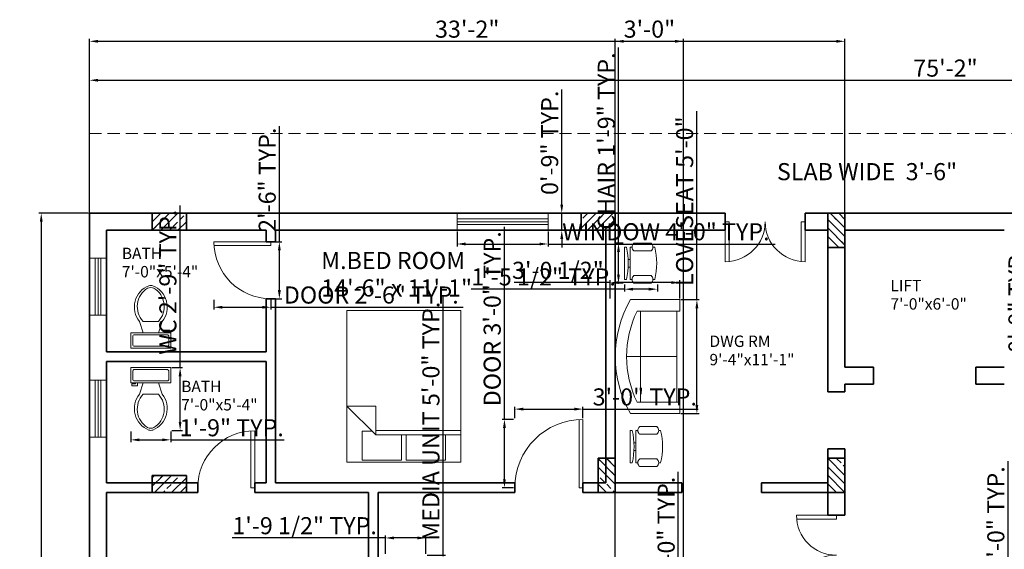
# Model space of a CAD drawing. Units: inches. Extents: x 2081 to 4786, y 1256 to 3802.
# Tile 5 of 7: x 2166 to 2685, y 1804 to 2083. Entities that reach past the tile are written whole.
import ezdxf

# ---------------------------------------------------------------- set-up
doc = ezdxf.new("R2010")
doc.units = ezdxf.units.IN
doc.linetypes.add('HIDDEN', pattern=[9.525, 6.35, -3.175])
for name, color, linetype, lineweight in [('A-ANNO-DIMS', 18, 'Continuous', 18), ('A-ANNO-TEXT', 18, 'Continuous', 18), ('A-AREA-IDEN', 18, 'Continuous', 18), ('A-COLS', 1, 'Continuous', 35), ('A-COLS-PATT', 1, 'Continuous', 13), ('A-DOOR', 5, 'Continuous', 18), ('A-FLOR-FIXT', 18, 'Continuous', 18), ('A-FLOR-OVHD', 18, 'HIDDEN', 18), ('A-FURN', 5, 'Continuous', 18), ('A-GLAZ', 11, 'Continuous', 18), ('A-WALL', 7, 'Continuous', 35)]:
    doc.layers.add(name, color=color, linetype=linetype, lineweight=lineweight)
doc.styles.get("Standard").update_dxf_attribs({"font": 'arial.ttf'})
doc.dimstyles.new('ISO-25', dxfattribs={"dimtxt": 9, "dimasz": 4.5, "dimexe": 1.25, "dimexo": 0.625, "dimtad": 1, "dimdec": 0, "dimlunit": 3, "dimtxsty": 'Standard', "dimcen": 2.5, "dimadec": 0, "dimazin": 0, "dimtfac": 1, "dimtdec": 0, "dimtmove": 0, "dimatfit": 3, "dimfxl": 1, "dimarcsym": 0})
pattern_1 = [(45, (-712.752, 64.734), (-13.47038, 13.47038), []), (45, (-708.262, 64.734), (-13.47038, 13.47038), []), (45, (-703.772, 64.734), (-13.47038, 13.47038), []), (45, (-699.281, 64.734), (-13.47038, 13.47038), [])]
pattern_2 = [(135, (1916.44, -3174.735), (-13.47038, -13.47038), []), (135, (1916.44, -3170.245), (-13.47038, -13.47038), []), (135, (1916.44, -3165.755), (-13.47038, -13.47038), []), (135, (1916.44, -3161.265), (-13.47038, -13.47038), [])]

# ---------------------------------------------------------------- blocks, each defined once
blk = doc.blocks.new('Sofa - Roundback Loveseat 5 ft.')
for p, q in [((0, -32.44198), (0, -5.99998)), ((-24, -33.99998), (-24, -11.46958)), ((-23.9998, -13.38178), (23.99986, -13.38178)), ((24.00004, -33.99998), (24.00004, -11.46958)), ((-24, -32.44198), (24.00004, -32.44198))]:
    blk.add_line(p, q)
for points in [[(-24, -33.99998), (-30, -33.99998), (-30, -7.99998)], [(30.00004, -7.99998), (30.00004, -33.99998), (24.00004, -33.99998)]]:
    blk.add_lwpolyline(points)
for centre, radius, start, end in [((0, -60.24998), 60.24998, 60.13715, 119.8628), ((0, -61.38438), 55.38444, 64.32083, 115.6792)]:
    blk.add_arc(centre, radius, start, end)
blk = doc.blocks.new('Bed - Queen')
for p, q in [((0, -80.00003), (0, 0)), ((0, 0), (59.99999, 0)), ((59.99999, 0), (59.99999, -80.00003)), ((7.99999, -1.2), (28.79998, -1.2)), ((7.99999, -14.4), (7.99999, -1.2)), ((28.79998, -1.2), (28.79998, -14.4)), ((31.19999, -1.2), (51.99999, -1.2)), ((31.19999, -14.4), (31.19999, -1.2)), ((51.99999, -1.2), (51.99999, -16.4)), ((0, -14.4), (44.8, -14.4)), ((59.99999, -29.6), (44.8, -14.4)), ((44.8, -14.4), (44.8, -29.6)), ((44.8, -16.8), (0, -16.8)), ((51.99999, -16.4), (46.79936, -16.4)), ((44.8, -29.6), (59.99999, -29.6)), ((59.99999, -80.00003), (0, -80.00003))]:
    blk.add_line(p, q)
blk = doc.blocks.new('Chair - Desk')
for p, q in [((-8.5, 0), (-8.5, -1)), ((-8.5, 0), (8.5, 0)), ((8.5, 0), (8.5, -1)), ((-10.5, -5), (-10.5, -14)), ((-8.5, -3), (-8.5, -4)), ((-8.5, -3), (8.5, -3)), ((-6.5, -14), (-6.5, -5)), ((-2, -3), (-2, -1.9355)), ((2, -1.9576), (2, -3)), ((6.5, -5), (6.5, -14)), ((8.5, -3), (8.5, -4)), ((10.5, -14), (10.5, -5)), ((-8.5, -15), (-8.5, -16)), ((8.5, -15), (8.5, -16))]:
    blk.add_line(p, q)
for centre, radius, start, end in [((-8.5, -6.5), 2.5, 36.8699, 143.1301), ((0, 34.625), 36.625, 256.5803, 283.4197), ((8.5, -6.5), 2.5, 36.8699, 143.1301), ((-8.5, -12.5), 2.5, 216.8699, 323.1301), ((8.5, -12.5), 2.5, 216.8699, 323.1301), ((0, 19.625), 36.625, 256.5803, 283.4197)]:
    blk.add_arc(centre, radius, start, end)
blk = doc.blocks.new('Toilet - top')
for p, q in [((9.5, -6), (9.5, -2)), ((-10, -8.5), (-8, -8.5)), ((-10, -9.5), (-10, -8.5)), ((-7, -9.5), (-10, -9.5)), ((-8, -8.5), (-8, -8)), ((-7, -8), (-7, -9.5)), ((-4, -8), (-6, -14)), ((4, -8), (6, -14)), ((4, -14), (-4, -14))]:
    blk.add_line(p, q)
blk.add_lwpolyline([(10.5, -8), (10.5, 0), (-10.5, 0), (-10.5, -8)], close=True)
for points in [[(-9.5, -2), (-9.5, -6)], [(8.5, -1), (-8.5, -1)], [(-8.5, -7), (8.5, -7)]]:
    blk.add_lwpolyline(points)
for centre, radius, start, end in [((-8.62, -1.88), 0.884, 81.8699, 188.1301), ((8.62, -1.88), 0.884, 351.8699, 98.1301), ((-8.62, -6.12), 0.884, 171.8699, 278.1301), ((8.62, -6.12), 0.884, 261.8699, 8.1301), ((3.52, -21.58), 12.17, 141.4691, 247.9714), ((4.2, -21.82), 11.33, 136.3677, 238.9468), ((-3.52, -21.58), 12.17, 292.0284, 38.5307), ((-4.2, -21.82), 11.33, 301.053, 43.6321), ((0, -27.88), 4, 245.7318, 294.2682), ((0, -29), 4, 254.8605, 285.1395)]:
    blk.add_arc(centre, radius, start, end)
blk = doc.blocks.new('*D23')
at = {"layer": 'A-ANNO-DIMS', "color": 0, "lineweight": -2, "transparency": 16777216}
for p, q in [((2202.98, 2023.8), (2202.98, 2052.41)), ((2207.48, 2051.16), (3100.48, 2051.16)), ((3104.98, 2023.8), (3104.98, 2052.41))]:
    blk.add_line(p, q, dxfattribs=at)
at = {"layer": 'A-ANNO-DIMS', "color": 0, "transparency": 16777216}
for points in [[(2207.48, 2051.91), (2207.48, 2050.41), (2202.98, 2051.16)], [(3100.48, 2051.91), (3100.48, 2050.41), (3104.98, 2051.16)]]:
    blk.add_solid(points, dxfattribs=at)
at = {"layer": 'Defpoints', "color": 0, "transparency": 16777216}
for p in [(3104.98, 2051.16), (2202.98, 2023.17), (3104.98, 2023.17)]:
    blk.add_point(p, dxfattribs=at)
at = {"layer": 'A-ANNO-DIMS', "color": 0, "transparency": 16777216, "insert": (2653.98, 2056.38), "char_height": 9, "attachment_point": 5}
blk.add_mtext('75\'-2"', dxfattribs=at)
blk = doc.blocks.new('*D25')
at = {"layer": 'A-ANNO-DIMS', "color": 0, "lineweight": -2, "transparency": 16777216}
for p, q in [((2202.36, 1981.17), (2176.26, 1981.17)), ((2177.51, 1976.67), (2177.51, 1437.67)), ((2202.36, 1433.17), (2176.26, 1433.17))]:
    blk.add_line(p, q, dxfattribs=at)
at = {"layer": 'A-ANNO-DIMS', "color": 0, "transparency": 16777216}
for points in [[(2176.76, 1976.67), (2178.26, 1976.67), (2177.51, 1981.17)], [(2176.76, 1437.67), (2178.26, 1437.67), (2177.51, 1433.17)]]:
    blk.add_solid(points, dxfattribs=at)
at = {"layer": 'Defpoints', "color": 0, "transparency": 16777216}
for p in [(2202.98, 1981.17), (2177.51, 1433.17), (2202.98, 1433.17)]:
    blk.add_point(p, dxfattribs=at)
at = {"layer": 'A-ANNO-DIMS', "color": 0, "transparency": 16777216, "insert": (2172.29, 1707.17), "char_height": 9, "attachment_point": 5, "rotation": 90}
blk.add_mtext('45\'-8"', dxfattribs=at)
blk = doc.blocks.new('DOOR-PAIR-42IN')
for p, q in [((0, 42), (21, 42)), ((21, 42), (21, 40)), ((0, 40), (21, 40)), ((0, 2), (21, 2)), ((21, 0), (21, 2)), ((0, 0), (21, 0))]:
    blk.add_line(p, q)
for centre, start, end in [((21, 42), 180, 270), ((21, 0), 90, 180)]:
    blk.add_arc(centre, 21, start, end)
blk = doc.blocks.new('DOOR-SINGLE-36IN')
for p, q in [((34, 36), (34, 0)), ((36, 36), (36, 0)), ((36, 0), (34, 0))]:
    blk.add_line(p, q)
blk.add_arc((36, 0), 36, 90, 180)
blk = doc.blocks.new('DOOR-SINGLE-30IN')
for p, q in [((0, 30), (30, 30)), ((0, 28), (30, 28)), ((30, 30), (30, 28))]:
    blk.add_line(p, q)
blk.add_arc((30, 30), 30, 180, 270)
blk = doc.blocks.new('WINDOW-48IN')
for p, q in [((0, 0), (0, 9)), ((0, 9), (4, 9)), ((48, 6), (0, 6)), ((4, 9), (48, 9)), ((48, 0), (48, 9)), ((48, 4.5), (0, 4.5)), ((48, 3), (0, 3)), ((48, 0), (0, 0))]:
    blk.add_line(p, q)
blk = doc.blocks.new('WINDOW-30IN')
for p, q in [((0, 0), (0, 30)), ((0, 30), (9, 30)), ((3, 0), (3, 30)), ((4.5, 0), (4.5, 30)), ((6, 0), (6, 30)), ((9, 30), (9, 0)), ((9, 0), (0, 0))]:
    blk.add_line(p, q)
blk = doc.blocks.new('COLUMN-9X18IN')
h = blk.add_hatch()
h.set_pattern_fill('ANSI34', color=256, angle=90)
h.set_pattern_definition(pattern_2)
h.paths.add_polyline_path([(9, 18), (0, 18), (0, 0), (9, 0)])
h = blk.add_hatch()
h.set_pattern_fill('ANSI34', color=256, angle=90)
h.set_pattern_definition(pattern_2)
h.paths.add_polyline_path([(9, 18), (0, 18), (0, 0), (9, 0)])
h = blk.add_hatch()
h.set_pattern_fill('ANSI34', color=256, angle=90)
h.set_pattern_definition(pattern_2)
h.paths.add_polyline_path([(9, 18), (0, 18), (0, 0), (9, 0)])
h = blk.add_hatch()
h.set_pattern_fill('ANSI33', color=256, angle=90)
h.set_pattern_definition([(135, (1916.44, -3174.7355), (-4.490128, -4.490128), []), (135, (1916.44, -3170.2454), (-4.490128, -4.490128), [3.175, -1.5875])])
h.paths.add_polyline_path([(0, 0), (9, 0), (9, 18), (0, 18)])
for p, q in [((0, 0), (0, 18)), ((0, 18), (9, 18)), ((9, 18), (9, 0)), ((9, 0), (0, 0))]:
    blk.add_line(p, q)
blk = doc.blocks.new('*D35')
at = {"layer": 'A-ANNO-DIMS', "color": 0, "lineweight": -2, "transparency": 16777216}
for p, q in [((2396.59, 1971.55), (2396.59, 1963.72)), ((2444.59, 1971.55), (2444.59, 1963.72)), ((2401.09, 1964.97), (2440.09, 1964.97)), ((2444.59, 1964.97), (2564.22, 1964.97))]:
    blk.add_line(p, q, dxfattribs=at)
at = {"layer": 'A-ANNO-DIMS', "color": 0, "transparency": 16777216}
for points in [[(2401.09, 1965.72), (2401.09, 1964.22), (2396.59, 1964.97)], [(2440.09, 1965.72), (2440.09, 1964.22), (2444.59, 1964.97)]]:
    blk.add_solid(points, dxfattribs=at)
at = {"layer": 'Defpoints', "color": 0, "transparency": 16777216}
for p in [(2396.59, 1972.17), (2444.59, 1972.17), (2444.59, 1964.97)]:
    blk.add_point(p, dxfattribs=at)
at = {"layer": 'A-ANNO-DIMS', "color": 0, "transparency": 16777216, "insert": (2506.66, 1970.25), "char_height": 9, "attachment_point": 5}
blk.add_mtext('WINDOW 4\'-0" TYP.', dxfattribs=at)
blk = doc.blocks.new('*D36')
at = {"layer": 'A-ANNO-DIMS', "color": 0, "lineweight": -2, "transparency": 16777216}
for p, q in [((2451.79, 1985.67), (2451.79, 2046.28)), ((2445.21, 1981.17), (2453.04, 1981.17)), ((2451.79, 1972.17), (2451.79, 1981.17)), ((2445.21, 1972.17), (2453.04, 1972.17)), ((2451.79, 1967.67), (2451.79, 1963.17))]:
    blk.add_line(p, q, dxfattribs=at)
at = {"layer": 'A-ANNO-DIMS', "color": 0, "transparency": 16777216}
for points in [[(2451.04, 1985.67), (2452.54, 1985.67), (2451.79, 1981.17)], [(2451.04, 1967.67), (2452.54, 1967.67), (2451.79, 1972.17)]]:
    blk.add_solid(points, dxfattribs=at)
at = {"layer": 'Defpoints', "color": 0, "transparency": 16777216}
for p in [(2444.59, 1981.17), (2451.79, 1981.17), (2444.59, 1972.17)]:
    blk.add_point(p, dxfattribs=at)
at = {"layer": 'A-ANNO-DIMS', "color": 0, "transparency": 16777216, "insert": (2446.57, 2018.23), "char_height": 9, "attachment_point": 5, "rotation": 90}
blk.add_mtext('0\'-9" TYP.', dxfattribs=at)
blk = doc.blocks.new('*D39')
at = {"layer": 'A-ANNO-DIMS', "color": 0, "lineweight": -2, "transparency": 16777216}
for p, q in [((2421.58, 1872.67), (2421.58, 1974.05)), ((2426.36, 1872.67), (2420.33, 1872.67)), ((2421.58, 1841.17), (2421.58, 1868.17)), ((2426.36, 1836.67), (2420.33, 1836.67))]:
    blk.add_line(p, q, dxfattribs=at)
at = {"layer": 'A-ANNO-DIMS', "color": 0, "transparency": 16777216}
for points in [[(2420.83, 1868.17), (2422.33, 1868.17), (2421.58, 1872.67)], [(2420.83, 1841.17), (2422.33, 1841.17), (2421.58, 1836.67)]]:
    blk.add_solid(points, dxfattribs=at)
at = {"layer": 'Defpoints', "color": 0, "transparency": 16777216}
for p in [(2421.58, 1872.67), (2426.98, 1872.67), (2426.98, 1836.67)]:
    blk.add_point(p, dxfattribs=at)
at = {"layer": 'A-ANNO-DIMS', "color": 0, "transparency": 16777216, "insert": (2416.3, 1925.61), "char_height": 9, "attachment_point": 5, "rotation": 90}
blk.add_mtext('DOOR 3\'-0" TYP.', dxfattribs=at)
blk = doc.blocks.new('*D40')
at = {"layer": 'A-ANNO-DIMS', "color": 0, "lineweight": -2, "transparency": 16777216}
for p, q in [((2426.98, 1873.3), (2426.98, 1879.32)), ((2462.98, 1873.3), (2462.98, 1879.32)), ((2431.48, 1878.07), (2458.48, 1878.07)), ((2462.98, 1878.07), (2523.59, 1878.07))]:
    blk.add_line(p, q, dxfattribs=at)
at = {"layer": 'A-ANNO-DIMS', "color": 0, "transparency": 16777216}
for points in [[(2431.48, 1878.82), (2431.48, 1877.32), (2426.98, 1878.07)], [(2458.48, 1878.82), (2458.48, 1877.32), (2462.98, 1878.07)]]:
    blk.add_solid(points, dxfattribs=at)
at = {"layer": 'Defpoints', "color": 0, "transparency": 16777216}
for p in [(2462.98, 1878.07), (2426.98, 1872.67), (2462.98, 1872.67)]:
    blk.add_point(p, dxfattribs=at)
at = {"layer": 'A-ANNO-DIMS', "color": 0, "transparency": 16777216, "insert": (2495.54, 1883.3), "char_height": 9, "attachment_point": 5}
blk.add_mtext('3\'-0" TYP.', dxfattribs=at)
blk = doc.blocks.new('*D41')
at = {"layer": 'A-ANNO-DIMS', "color": 0, "lineweight": -2, "transparency": 16777216}
for p, q in [((2250.68, 1899.88), (2250.68, 1985.3)), ((2246.35, 1899.88), (2251.93, 1899.88)), ((2250.68, 1871.33), (2250.68, 1895.38)), ((2246.35, 1866.83), (2251.93, 1866.83))]:
    blk.add_line(p, q, dxfattribs=at)
at = {"layer": 'A-ANNO-DIMS', "color": 0, "transparency": 16777216}
for points in [[(2249.93, 1895.38), (2251.43, 1895.38), (2250.68, 1899.88)], [(2249.93, 1871.33), (2251.43, 1871.33), (2250.68, 1866.83)]]:
    blk.add_solid(points, dxfattribs=at)
at = {"layer": 'Defpoints', "color": 0, "transparency": 16777216}
for p in [(2245.73, 1899.88), (2250.68, 1899.88), (2245.73, 1866.83)]:
    blk.add_point(p, dxfattribs=at)
at = {"layer": 'A-ANNO-DIMS', "color": 0, "transparency": 16777216, "insert": (2245.4, 1944.84), "char_height": 9, "attachment_point": 5, "rotation": 90}
blk.add_mtext('WC 2\'-9" TYP.', dxfattribs=at)
blk = doc.blocks.new('*D42')
at = {"layer": 'A-ANNO-DIMS', "color": 0, "lineweight": -2, "transparency": 16777216}
for p, q in [((2224.73, 1866.21), (2224.73, 1860.63)), ((2245.73, 1866.21), (2245.73, 1860.63)), ((2229.23, 1861.88), (2241.23, 1861.88)), ((2245.73, 1861.88), (2305.49, 1861.88))]:
    blk.add_line(p, q, dxfattribs=at)
at = {"layer": 'A-ANNO-DIMS', "color": 0, "transparency": 16777216}
for points in [[(2229.23, 1862.63), (2229.23, 1861.13), (2224.73, 1861.88)], [(2241.23, 1862.63), (2241.23, 1861.13), (2245.73, 1861.88)]]:
    blk.add_solid(points, dxfattribs=at)
at = {"layer": 'Defpoints', "color": 0, "transparency": 16777216}
for p in [(2224.73, 1866.83), (2245.73, 1866.83), (2245.73, 1861.88)]:
    blk.add_point(p, dxfattribs=at)
at = {"layer": 'A-ANNO-DIMS', "color": 0, "transparency": 16777216, "insert": (2277.86, 1867.1), "char_height": 9, "attachment_point": 5}
blk.add_mtext('1\'-9" TYP.', dxfattribs=at)
blk = doc.blocks.new('*D45')
at = {"layer": 'A-ANNO-DIMS', "color": 0, "lineweight": -2, "transparency": 16777216}
for p, q in [((2268.48, 1935.55), (2268.48, 1930.42)), ((2298.48, 1935.55), (2298.48, 1930.42)), ((2272.98, 1931.67), (2293.98, 1931.67)), ((2298.48, 1931.67), (2399.86, 1931.67))]:
    blk.add_line(p, q, dxfattribs=at)
at = {"layer": 'A-ANNO-DIMS', "color": 0, "transparency": 16777216}
for points in [[(2272.98, 1932.42), (2272.98, 1930.92), (2268.48, 1931.67)], [(2293.98, 1932.42), (2293.98, 1930.92), (2298.48, 1931.67)]]:
    blk.add_solid(points, dxfattribs=at)
at = {"layer": 'Defpoints', "color": 0, "transparency": 16777216}
for p in [(2268.48, 1936.17), (2298.48, 1936.17), (2298.48, 1931.67)]:
    blk.add_point(p, dxfattribs=at)
at = {"layer": 'A-ANNO-DIMS', "color": 0, "transparency": 16777216, "insert": (2351.42, 1936.95), "char_height": 9, "attachment_point": 5}
blk.add_mtext('DOOR 2\'-6" TYP.', dxfattribs=at)
blk = doc.blocks.new('*D46')
at = {"layer": 'A-ANNO-DIMS', "color": 0, "lineweight": -2, "transparency": 16777216}
for p, q in [((2302.98, 1966.17), (2302.98, 2026.94)), ((2299.11, 1966.17), (2304.23, 1966.17)), ((2302.98, 1940.67), (2302.98, 1961.67)), ((2299.11, 1936.17), (2304.23, 1936.17))]:
    blk.add_line(p, q, dxfattribs=at)
at = {"layer": 'A-ANNO-DIMS', "color": 0, "transparency": 16777216}
for points in [[(2302.23, 1961.67), (2303.73, 1961.67), (2302.98, 1966.17)], [(2302.23, 1940.67), (2303.73, 1940.67), (2302.98, 1936.17)]]:
    blk.add_solid(points, dxfattribs=at)
at = {"layer": 'Defpoints', "color": 0, "transparency": 16777216}
for p in [(2298.48, 1966.17), (2302.98, 1966.17), (2298.48, 1936.17)]:
    blk.add_point(p, dxfattribs=at)
at = {"layer": 'A-ANNO-DIMS', "color": 0, "transparency": 16777216, "insert": (2297.76, 1998.8), "char_height": 9, "attachment_point": 5, "rotation": 90}
blk.add_mtext('2\'-6" TYP.', dxfattribs=at)
blk = doc.blocks.new('*D48')
at = {"layer": 'A-ANNO-DIMS', "color": 0, "lineweight": -2, "transparency": 16777216}
for p, q in [((2698.02, 1985.67), (2698.02, 1990.17)), ((2701.9, 1981.17), (2696.77, 1981.17)), ((2698.02, 1981.17), (2698.02, 1972.17)), ((2701.9, 1972.17), (2696.77, 1972.17)), ((2698.02, 1967.67), (2698.02, 1907.06))]:
    blk.add_line(p, q, dxfattribs=at)
at = {"layer": 'A-ANNO-DIMS', "color": 0, "transparency": 16777216}
for points in [[(2697.27, 1985.67), (2698.77, 1985.67), (2698.02, 1981.17)], [(2697.27, 1967.67), (2698.77, 1967.67), (2698.02, 1972.17)]]:
    blk.add_solid(points, dxfattribs=at)
at = {"layer": 'Defpoints', "color": 0, "transparency": 16777216}
for p in [(2702.52, 1981.17), (2698.02, 1972.17), (2702.52, 1972.17)]:
    blk.add_point(p, dxfattribs=at)
at = {"layer": 'A-ANNO-DIMS', "color": 0, "transparency": 16777216, "insert": (2692.8, 1935.12), "char_height": 9, "attachment_point": 5, "rotation": 90}
blk.add_mtext('0\'-9" TYP.', dxfattribs=at)
blk = doc.blocks.new('*D49')
at = {"layer": 'A-ANNO-DIMS', "color": 0, "lineweight": -2, "transparency": 16777216}
for p, q in [((2481.68, 1965.34), (2481.68, 2068.46)), ((2484.21, 1965.34), (2480.43, 1965.34)), ((2481.68, 1948.84), (2481.68, 1960.84)), ((2484.21, 1944.34), (2480.43, 1944.34))]:
    blk.add_line(p, q, dxfattribs=at)
at = {"layer": 'A-ANNO-DIMS', "color": 0, "transparency": 16777216}
for points in [[(2480.93, 1960.84), (2482.43, 1960.84), (2481.68, 1965.34)], [(2480.93, 1948.84), (2482.43, 1948.84), (2481.68, 1944.34)]]:
    blk.add_solid(points, dxfattribs=at)
at = {"layer": 'Defpoints', "color": 0, "transparency": 16777216}
for p in [(2481.68, 1965.34), (2484.83, 1965.34), (2484.83, 1944.34)]:
    blk.add_point(p, dxfattribs=at)
at = {"layer": 'A-ANNO-DIMS', "color": 0, "transparency": 16777216, "insert": (2476.4, 2019.15), "char_height": 9, "attachment_point": 5, "rotation": 90}
blk.add_mtext('CHAIR 1\'-9" TYP.', dxfattribs=at)
blk = doc.blocks.new('*D50')
at = {"layer": 'A-ANNO-DIMS', "color": 0, "lineweight": -2, "transparency": 16777216}
for p, q in [((2484.83, 1941.19), (2404.1, 1941.19)), ((2484.83, 1943.72), (2484.83, 1939.94)), ((2497.66, 1941.19), (2489.33, 1941.19)), ((2502.16, 1943.72), (2502.16, 1939.94))]:
    blk.add_line(p, q, dxfattribs=at)
at = {"layer": 'A-ANNO-DIMS', "color": 0, "transparency": 16777216}
for points in [[(2489.33, 1941.94), (2489.33, 1940.44), (2484.83, 1941.19)], [(2497.66, 1941.94), (2497.66, 1940.44), (2502.16, 1941.19)]]:
    blk.add_solid(points, dxfattribs=at)
at = {"layer": 'Defpoints', "color": 0, "transparency": 16777216}
for p in [(2484.83, 1944.34), (2484.83, 1941.19), (2502.16, 1944.34)]:
    blk.add_point(p, dxfattribs=at)
at = {"layer": 'A-ANNO-DIMS', "color": 0, "transparency": 16777216, "insert": (2442.21, 1946.47), "char_height": 9, "attachment_point": 5}
blk.add_mtext('1\'-5 1/2" TYP.', dxfattribs=at)
blk = doc.blocks.new('*D55')
at = {"layer": 'A-ANNO-DIMS', "color": 0, "lineweight": -2, "transparency": 16777216}
for p, q in [((2686.95, 1752.41), (2686.95, 1850.7)), ((2698.93, 1752.41), (2685.7, 1752.41)), ((2686.95, 1672.91), (2686.95, 1747.91)), ((2698.93, 1668.41), (2685.7, 1668.41))]:
    blk.add_line(p, q, dxfattribs=at)
at = {"layer": 'A-ANNO-DIMS', "color": 0, "transparency": 16777216}
for points in [[(2686.2, 1747.91), (2687.7, 1747.91), (2686.95, 1752.41)], [(2686.2, 1672.91), (2687.7, 1672.91), (2686.95, 1668.41)]]:
    blk.add_solid(points, dxfattribs=at)
at = {"layer": 'Defpoints', "color": 0, "transparency": 16777216}
for p in [(2686.95, 1752.41), (2699.55, 1752.41), (2699.55, 1668.41)]:
    blk.add_point(p, dxfattribs=at)
at = {"layer": 'A-ANNO-DIMS', "color": 0, "transparency": 16777216, "insert": (2681.67, 1803.8), "char_height": 9, "attachment_point": 5, "rotation": 90}
blk.add_mtext('SOFA 7\'-0" TYP.', dxfattribs=at)
blk = doc.blocks.new('*D57')
at = {"layer": 'A-ANNO-DIMS', "color": 0, "lineweight": -2, "transparency": 16777216}
for p, q in [((2513.19, 1740.9), (2513.19, 1845.06)), ((2521.57, 1740.9), (2511.94, 1740.9)), ((2513.19, 1685.4), (2513.19, 1736.4)), ((2521.57, 1680.9), (2511.94, 1680.9))]:
    blk.add_line(p, q, dxfattribs=at)
at = {"layer": 'A-ANNO-DIMS', "color": 0, "transparency": 16777216}
for points in [[(2512.44, 1736.4), (2513.94, 1736.4), (2513.19, 1740.9)], [(2512.44, 1685.4), (2513.94, 1685.4), (2513.19, 1680.9)]]:
    blk.add_solid(points, dxfattribs=at)
at = {"layer": 'Defpoints', "color": 0, "transparency": 16777216}
for p in [(2513.19, 1740.9), (2522.19, 1740.9), (2522.19, 1680.9)]:
    blk.add_point(p, dxfattribs=at)
at = {"layer": 'A-ANNO-DIMS', "color": 0, "transparency": 16777216, "insert": (2507.97, 1795.23), "char_height": 9, "attachment_point": 5, "rotation": 90}
blk.add_mtext('TABLE 5\'-0" TYP.', dxfattribs=at)
blk = doc.blocks.new('*D59')
at = {"layer": 'A-ANNO-DIMS', "color": 0, "lineweight": -2, "transparency": 16777216}
for p, q in [((2389.23, 1801.25), (2389.23, 1937.59)), ((2380.85, 1801.25), (2390.48, 1801.25)), ((2389.23, 1745.75), (2389.23, 1796.75)), ((2380.85, 1741.25), (2390.48, 1741.25))]:
    blk.add_line(p, q, dxfattribs=at)
at = {"layer": 'A-ANNO-DIMS', "color": 0, "transparency": 16777216}
for points in [[(2388.48, 1796.75), (2389.98, 1796.75), (2389.23, 1801.25)], [(2388.48, 1745.75), (2389.98, 1745.75), (2389.23, 1741.25)]]:
    blk.add_solid(points, dxfattribs=at)
at = {"layer": 'Defpoints', "color": 0, "transparency": 16777216}
for p in [(2380.23, 1801.25), (2389.23, 1801.25), (2380.23, 1741.25)]:
    blk.add_point(p, dxfattribs=at)
at = {"layer": 'A-ANNO-DIMS', "color": 0, "transparency": 16777216, "insert": (2384.01, 1871.67), "char_height": 9, "attachment_point": 5, "rotation": 90}
blk.add_mtext('MEDIA UNIT 5\'-0" TYP.', dxfattribs=at)
blk = doc.blocks.new('*D60')
at = {"layer": 'A-ANNO-DIMS', "color": 0, "lineweight": -2, "transparency": 16777216}
for p, q in [((2358.89, 1801.88), (2358.89, 1811.5)), ((2380.23, 1801.88), (2380.23, 1811.5)), ((2358.89, 1810.25), (2278.16, 1810.25)), ((2375.73, 1810.25), (2363.39, 1810.25))]:
    blk.add_line(p, q, dxfattribs=at)
at = {"layer": 'A-ANNO-DIMS', "color": 0, "transparency": 16777216}
for points in [[(2363.39, 1811), (2363.39, 1809.5), (2358.89, 1810.25)], [(2375.73, 1811), (2375.73, 1809.5), (2380.23, 1810.25)]]:
    blk.add_solid(points, dxfattribs=at)
at = {"layer": 'Defpoints', "color": 0, "transparency": 16777216}
for p in [(2358.89, 1810.25), (2358.89, 1801.25), (2380.23, 1801.25)]:
    blk.add_point(p, dxfattribs=at)
at = {"layer": 'A-ANNO-DIMS', "color": 0, "transparency": 16777216, "insert": (2316.28, 1815.53), "char_height": 9, "attachment_point": 5}
blk.add_mtext('1\'-9 1/2" TYP.', dxfattribs=at)
blk = doc.blocks.new('*D73')
at = {"layer": 'A-ANNO-DIMS', "color": 0, "lineweight": -2, "transparency": 16777216}
for p, q in [((2522.98, 1935.67), (2522.98, 2034.82)), ((2514.61, 1935.67), (2524.23, 1935.67)), ((2522.98, 1880.17), (2522.98, 1931.17)), ((2514.61, 1875.67), (2524.23, 1875.67))]:
    blk.add_line(p, q, dxfattribs=at)
at = {"layer": 'A-ANNO-DIMS', "color": 0, "transparency": 16777216}
for points in [[(2522.23, 1931.17), (2523.73, 1931.17), (2522.98, 1935.67)], [(2522.23, 1880.17), (2523.73, 1880.17), (2522.98, 1875.67)]]:
    blk.add_solid(points, dxfattribs=at)
at = {"layer": 'Defpoints', "color": 0, "transparency": 16777216}
for p in [(2513.98, 1935.67), (2522.98, 1935.67), (2513.98, 1875.67)]:
    blk.add_point(p, dxfattribs=at)
at = {"layer": 'A-ANNO-DIMS', "color": 0, "transparency": 16777216, "insert": (2517.7, 1987.5), "char_height": 9, "attachment_point": 5, "rotation": 90}
blk.add_mtext('LOVESEAT 5\'-0"', dxfattribs=at)
blk = doc.blocks.new('*D74')
at = {"layer": 'A-ANNO-DIMS', "color": 0, "lineweight": -2, "transparency": 16777216}
for p, q in [((2477.32, 1936.3), (2477.32, 1945.92)), ((2513.98, 1936.3), (2513.98, 1945.92)), ((2477.32, 1944.67), (2426.68, 1944.67)), ((2509.48, 1944.67), (2481.82, 1944.67))]:
    blk.add_line(p, q, dxfattribs=at)
at = {"layer": 'A-ANNO-DIMS', "color": 0, "transparency": 16777216}
for points in [[(2481.82, 1945.42), (2481.82, 1943.92), (2477.32, 1944.67)], [(2509.48, 1945.42), (2509.48, 1943.92), (2513.98, 1944.67)]]:
    blk.add_solid(points, dxfattribs=at)
at = {"layer": 'Defpoints', "color": 0, "transparency": 16777216}
for p in [(2477.32, 1944.67), (2477.32, 1935.67), (2513.98, 1935.67)]:
    blk.add_point(p, dxfattribs=at)
at = {"layer": 'A-ANNO-DIMS', "color": 0, "transparency": 16777216, "insert": (2449.75, 1949.95), "char_height": 9, "attachment_point": 5}
blk.add_mtext('3\'-0 1/2"', dxfattribs=at)
blk = doc.blocks.new('*D77')
at = {"layer": 'A-ANNO-DIMS', "color": 0, "lineweight": -2, "transparency": 16777216}
for p, q in [((2202.98, 1981.8), (2202.98, 2072.92)), ((2207.48, 2071.67), (2596.48, 2071.67)), ((2600.98, 1981.8), (2600.98, 2072.92))]:
    blk.add_line(p, q, dxfattribs=at)
at = {"layer": 'A-ANNO-DIMS', "color": 0, "transparency": 16777216}
for points in [[(2207.48, 2072.42), (2207.48, 2070.92), (2202.98, 2071.67)], [(2596.48, 2072.42), (2596.48, 2070.92), (2600.98, 2071.67)]]:
    blk.add_solid(points, dxfattribs=at)
at = {"layer": 'Defpoints', "color": 0, "transparency": 16777216}
for p in [(2600.98, 2071.67), (2202.98, 1981.17), (2600.98, 1981.17)]:
    blk.add_point(p, dxfattribs=at)
at = {"layer": 'A-ANNO-DIMS', "color": 0, "transparency": 16777216, "insert": (2401.98, 2076.9), "char_height": 9, "attachment_point": 5}
blk.add_mtext('33\'-2"', dxfattribs=at)
blk = doc.blocks.new('*D78')
at = {"layer": 'A-ANNO-DIMS', "color": 0, "lineweight": -2, "transparency": 16777216}
for p, q in [((2479.98, 1626.8), (2479.98, 2072.92)), ((2484.48, 2071.67), (2511.48, 2071.67)), ((2515.98, 1639.8), (2515.98, 2072.92))]:
    blk.add_line(p, q, dxfattribs=at)
at = {"layer": 'A-ANNO-DIMS', "color": 0, "transparency": 16777216}
for points in [[(2484.48, 2072.42), (2484.48, 2070.92), (2479.98, 2071.67)], [(2511.48, 2072.42), (2511.48, 2070.92), (2515.98, 2071.67)]]:
    blk.add_solid(points, dxfattribs=at)
at = {"layer": 'Defpoints', "color": 0, "transparency": 16777216}
for p in [(2515.98, 2071.67), (2515.98, 1639.17), (2479.98, 1626.17)]:
    blk.add_point(p, dxfattribs=at)
at = {"layer": 'A-ANNO-DIMS', "color": 0, "transparency": 16777216, "insert": (2497.98, 2076.9), "char_height": 9, "attachment_point": 5}
blk.add_mtext('3\'-0"', dxfattribs=at)

msp = doc.modelspace()

# ---------------------------------------------------------------- hatches: boundary and pattern name
at = {"layer": 'A-COLS-PATT'}
h = msp.add_hatch(dxfattribs=at)
h.set_pattern_fill('ANSI34', color=256)
h.set_pattern_definition(pattern_1)
h.paths.add_polyline_path([(2479.98, 1981.17), (2461.98, 1981.17), (2461.98, 1972.17), (2479.98, 1972.17)])
h = msp.add_hatch(dxfattribs=at)
h.set_pattern_fill('ANSI34', color=256)
h.set_pattern_definition(pattern_1)
h.paths.add_polyline_path([(2479.98, 1981.17), (2461.98, 1981.17), (2461.98, 1972.17), (2479.98, 1972.17)])
h = msp.add_hatch(dxfattribs=at)
h.set_pattern_fill('ANSI34', color=256)
h.set_pattern_definition(pattern_1)
h.paths.add_polyline_path([(2479.98, 1981.17), (2461.98, 1981.17), (2461.98, 1972.17), (2479.98, 1972.17)])
h = msp.add_hatch(dxfattribs=at)
h.set_pattern_fill('ANSI33', color=256)
h.set_pattern_definition([(45, (-712.752, 64.7335), (-4.490128, 4.490128), []), (45, (-708.262, 64.7335), (-4.490128, 4.490128), [3.175, -1.5875])])
h.paths.add_polyline_path([(2479.98, 1981.17), (2461.98, 1981.17), (2461.98, 1972.17), (2479.98, 1972.17)])

# ---------------------------------------------------------------- linework, layer by layer
at = {"layer": 'A-COLS'}
for p, q in [((2461.98, 1981.17), (2479.98, 1981.17)), ((2461.98, 1972.17), (2461.98, 1981.17)), ((2479.98, 1981.17), (2479.98, 1972.17)), ((2479.98, 1972.17), (2461.98, 1972.17))]:
    msp.add_line(p, q, dxfattribs=at)
at = {"layer": 'A-FLOR-OVHD'}
for p, q in [((2202.98, 1981.17), (2202.98, 2023.17)), ((2202.98, 2023.17), (3062.98, 2023.17))]:
    msp.add_line(p, q, dxfattribs=at)
at = {"layer": 'A-WALL'}
for p, q in [((2202.98, 1981.17), (2537.98, 1981.17)), ((2202.98, 1981.17), (2202.98, 1433.17)), ((2537.98, 1972.17), (2537.98, 1981.17)), ((2579.98, 1981.17), (2987.98, 1981.17)), ((2579.98, 1972.17), (2579.98, 1981.17)), ((2211.98, 1972.17), (2295.98, 1972.17)), ((2211.98, 1908.17), (2211.98, 1972.17)), ((2295.98, 1966.17), (2295.98, 1972.17)), ((2300.98, 1966.17), (2300.98, 1972.17)), ((2300.98, 1972.17), (2474.98, 1972.17)), ((2474.98, 1839.17), (2474.98, 1972.17)), ((2479.98, 1839.17), (2479.98, 1972.17)), ((2479.98, 1972.17), (2537.98, 1972.17)), ((2579.98, 1972.17), (2591.98, 1972.17)), ((2591.98, 1887.17), (2591.98, 1972.17)), ((2600.98, 1972.17), (2684.98, 1972.17)), ((2600.98, 1900.17), (2600.98, 1972.17)), ((2295.98, 1966.17), (2300.98, 1966.17)), ((2295.98, 1936.17), (2300.98, 1936.17)), ((2295.98, 1908.17), (2295.98, 1936.17)), ((2300.98, 1839.17), (2300.98, 1936.17)), ((2211.98, 1908.17), (2295.98, 1908.17)), ((2211.98, 1903.17), (2295.98, 1903.17)), ((2211.98, 1839.17), (2211.98, 1903.17)), ((2295.98, 1839.17), (2295.98, 1903.17)), ((2600.98, 1900.17), (2615.98, 1900.17)), ((2615.98, 1891.17), (2615.98, 1900.17)), ((2669.98, 1900.17), (2684.98, 1900.17)), ((2669.98, 1891.17), (2669.98, 1900.17)), ((2600.98, 1887.17), (2600.98, 1891.17)), ((2600.98, 1891.17), (2615.98, 1891.17)), ((2669.98, 1891.17), (2684.98, 1891.17)), ((2591.98, 1887.17), (2600.98, 1887.17)), ((2591.98, 1857.17), (2600.98, 1857.17)), ((2591.98, 1839.17), (2591.98, 1857.17)), ((2600.98, 1822.17), (2600.98, 1857.17)), ((2211.98, 1839.17), (2259.98, 1839.17)), ((2259.98, 1839.17), (2259.98, 1834.17)), ((2289.98, 1834.17), (2289.98, 1839.17)), ((2289.98, 1839.17), (2295.98, 1839.17)), ((2300.98, 1839.17), (2426.98, 1839.17)), ((2426.98, 1834.17), (2426.98, 1839.17)), ((2462.98, 1834.17), (2462.98, 1839.17)), ((2462.98, 1839.17), (2474.98, 1839.17)), ((2479.98, 1839.17), (2514.98, 1839.17)), ((2479.98, 1839.17), (2514.98, 1839.17)), ((2514.98, 1839.17), (2514.98, 1834.17)), ((2556.98, 1839.17), (2556.98, 1834.17)), ((2556.98, 1839.17), (2591.98, 1839.17)), ((2556.98, 1839.17), (2591.98, 1839.17)), ((2211.98, 1834.17), (2259.98, 1834.17)), ((2211.98, 1715.17), (2211.98, 1834.17)), ((2289.98, 1834.17), (2349.98, 1834.17)), ((2349.98, 1715.17), (2349.98, 1834.17)), ((2354.98, 1710.17), (2354.98, 1834.17)), ((2354.98, 1834.17), (2426.98, 1834.17)), ((2462.98, 1834.17), (2514.98, 1834.17)), ((2556.98, 1834.17), (2591.98, 1834.17)), ((2591.98, 1822.17), (2591.98, 1834.17)), ((2591.98, 1822.17), (2600.98, 1822.17))]:
    msp.add_line(p, q, dxfattribs=at)

# ---------------------------------------------------------------- block references
at = {"layer": 'A-COLS'}
for p, rotation in [((2235.98, 1981.17), 269.9999999999957), ((2235.98, 1843.17), 269.9999999999924)]:
    msp.add_blockref('COLUMN-9X18IN', p, dxfattribs=dict(at, rotation=rotation))
for p in [(2591.98, 1963.17), (2470.98, 1834.17), (2591.98, 1834.18)]:
    msp.add_blockref('COLUMN-9X18IN', p, dxfattribs=at)
at = {"layer": 'A-DOOR'}
for name, p, rotation in [('DOOR-PAIR-42IN', (2579.98, 1955.67), 90.00000000000058), ('DOOR-SINGLE-30IN', (2259.98, 1866.67), 270)]:
    msp.add_blockref(name, p, dxfattribs=dict(at, rotation=rotation))
for name, p in [('DOOR-SINGLE-30IN', (2268.48, 1936.17)), ('DOOR-SINGLE-36IN', (2426.98, 1836.67)), ('DOOR-PAIR-42IN', (2575.48, 1780.17))]:
    msp.add_blockref(name, p, dxfattribs=at)
at = {"layer": 'A-FLOR-FIXT', "rotation": 180}
msp.add_blockref('Toilet - top', (2235.23, 1910.17), dxfattribs=at)
at = {"layer": 'A-FLOR-FIXT'}
msp.add_blockref('Toilet - top', (2235.23, 1899.88), dxfattribs=at)
at = {"layer": 'A-FURN'}
for name, p, rotation in [('Chair - Desk', (2484.83, 1954.84), 90), ('Sofa - Roundback Loveseat 5 ft.', (2479.98, 1905.67), 90), ('Bed - Queen', (2398.53, 1850.05), 180), ('Chair - Desk', (2487.89, 1858.33), 90)]:
    msp.add_blockref(name, p, dxfattribs=dict(at, rotation=rotation))
at = {"layer": 'A-GLAZ'}
for name, p in [('WINDOW-48IN', (2396.59, 1972.17)), ('WINDOW-30IN', (2202.98, 1927.45)), ('WINDOW-30IN', (2202.98, 1863.37))]:
    msp.add_blockref(name, p, dxfattribs=at)

# ---------------------------------------------------------------- texts
at = {"layer": 'A-ANNO-TEXT'}
msp.add_text('SLAB WIDE  3\'-6"', height=9, dxfattribs=at).set_placement((2565.17, 1998.55))
at = {"layer": 'A-AREA-IDEN'}
for s, height, p in [('BATH', 6, (2219.98, 1957.02)), ('M.BED ROOM', 9, (2325.03, 1951.79)), ('7\'-0"x5\'-4"', 6, (2219.98, 1947.38)), ('14\'-6" x 11\'-1"', 9, (2325.03, 1937.33)), ('LIFT', 6, (2625, 1940.08)), ('7\'-0"x6\'-0"', 6, (2625, 1930.44)), ('DWG RM', 6, (2529.63, 1910.77)), ('9\'-4"x11\'-1"', 6, (2529.63, 1901.13)), ('BATH', 6, (2251.26, 1886.99)), ('7\'-0"x5\'-4"', 6, (2251.26, 1877.35))]:
    msp.add_text(s, height=height, dxfattribs=at).set_placement(p)

# ---------------------------------------------------------------- dimensions: what is measured, and where the dimension line sits
at = {"layer": 'A-ANNO-DIMS'}
for base, p1, p2, override, picture, middle in [((2600.98, 2071.67), (2202.98, 1981.17), (2600.98, 1981.17), {"dimdec": 1, "dimlfac": 1, "dimrnd": 0, "dimzin": 1, "dimdsep": 46, "dimlunit": 4, "dimfrac": 2}, '*D77', (2401.98, 2076.9)), ((2515.98, 2071.67), (2479.98, 1626.17), (2515.98, 1639.17), {"dimdec": 1, "dimlfac": 1, "dimrnd": 0, "dimzin": 1, "dimdsep": 46, "dimlunit": 4, "dimfrac": 2}, '*D78', (2497.98, 2076.9)), ((3104.98, 2051.16), (2202.98, 2023.17), (3104.98, 2023.17), {"dimclrd": 0, "dimclre": 0, "dimclrt": 0}, '*D23', (2653.98, 2056.38))]:
    dim = msp.add_linear_dim(base=base, p1=p1, p2=p2, dimstyle='ISO-25', override=override, dxfattribs=at)
    dim.commit()
    dim.dimension.update_dxf_attribs({"geometry": picture, "text_midpoint": middle})
for base, p1, p2, angle, text, picture, middle in [((2481.68, 1965.34), (2484.83, 1944.34), (2484.83, 1965.34), 90, 'CHAIR <> TYP.', '*D49', (2476.4, 2019.15)), ((2451.79, 1981.17), (2444.59, 1972.17), (2444.59, 1981.17), 90, '<> TYP.', '*D36', (2446.57, 2018.23)), ((2522.98, 1935.67), (2513.98, 1875.67), (2513.98, 1935.67), 90, 'LOVESEAT <>', '*D73', (2517.7, 1987.5)), ((2302.98, 1966.17), (2298.48, 1936.17), (2298.48, 1966.17), 90, '<> TYP.', '*D46', (2297.76, 1998.8)), ((2698.02, 1972.17), (2702.52, 1981.17), (2702.52, 1972.17), 270, '<> TYP.', '*D48', (2692.8, 1935.12)), ((2250.6827, 1899.8787), (2245.7258, 1866.8325), (2245.7258, 1899.8787), 90, 'WC <> TYP.', '*D41', (2245.4043, 1944.8377)), ((2421.58, 1872.67), (2426.98, 1836.67), (2426.98, 1872.67), 90, 'DOOR <> TYP.', '*D39', (2416.3, 1925.61)), ((2484.83, 1941.19), (2502.16, 1944.34), (2484.83, 1944.34), 180, '<> TYP.', '*D50', (2442.21, 1946.47)), ((2389.23, 1801.25), (2380.23, 1741.25), (2380.23, 1801.25), 90, 'MEDIA UNIT <> TYP.', '*D59', (2384.01, 1871.67)), ((2686.95, 1752.41), (2699.55, 1668.41), (2699.55, 1752.41), 90, 'SOFA <> TYP.', '*D55', (2681.67, 1803.8)), ((2513.19, 1740.9), (2522.19, 1680.9), (2522.19, 1740.9), 90, 'TABLE <> TYP.', '*D57', (2507.97, 1795.23)), ((2358.89, 1810.25), (2380.23, 1801.25), (2358.89, 1801.25), 180, '<> TYP.', '*D60', (2316.28, 1815.53))]:
    dim = msp.add_linear_dim(base=base, p1=p1, p2=p2, angle=angle, text=text, dimstyle='ISO-25', override={"dimdec": 1, "dimlfac": 1, "dimrnd": 0, "dimzin": 1, "dimdsep": 46, "dimlunit": 4, "dimfrac": 2}, dxfattribs=at)
    dim.commit()
    dim.dimension.update_dxf_attribs({"geometry": picture, "text_midpoint": middle})
for base, p1, p2, text, picture, middle in [((2444.59, 1964.97), (2396.59, 1972.17), (2444.59, 1972.17), 'WINDOW <> TYP.', '*D35', (2506.66, 1970.25)), ((2298.48, 1931.67), (2268.48, 1936.17), (2298.48, 1936.17), 'DOOR <> TYP.', '*D45', (2351.42, 1936.95)), ((2462.98, 1878.07), (2426.98, 1872.67), (2462.98, 1872.67), '<> TYP.', '*D40', (2495.54, 1883.3)), ((2245.73, 1861.88), (2224.73, 1866.83), (2245.73, 1866.83), '<> TYP.', '*D42', (2277.86, 1867.1))]:
    dim = msp.add_linear_dim(base=base, p1=p1, p2=p2, text=text, dimstyle='ISO-25', override={"dimdec": 1, "dimlfac": 1, "dimrnd": 0, "dimzin": 1, "dimdsep": 46, "dimlunit": 4, "dimfrac": 2}, dxfattribs=at)
    dim.commit()
    dim.dimension.update_dxf_attribs({"geometry": picture, "text_midpoint": middle})
for base, p1, p2, angle, override, picture, middle in [((2177.51, 1433.17), (2202.98, 1981.17), (2202.98, 1433.17), 90, {"dimclrd": 0, "dimclre": 0, "dimclrt": 0}, '*D25', (2172.29, 1707.17)), ((2477.32, 1944.67), (2513.98, 1935.67), (2477.32, 1935.67), 180, {"dimdec": 1, "dimlfac": 1, "dimrnd": 0, "dimzin": 1, "dimdsep": 46, "dimlunit": 4, "dimfrac": 2}, '*D74', (2449.75, 1949.95))]:
    dim = msp.add_linear_dim(base=base, p1=p1, p2=p2, angle=angle, dimstyle='ISO-25', override=override, dxfattribs=at)
    dim.commit()
    dim.dimension.update_dxf_attribs({"geometry": picture, "text_midpoint": middle})

doc.saveas('drawing.dxf')
